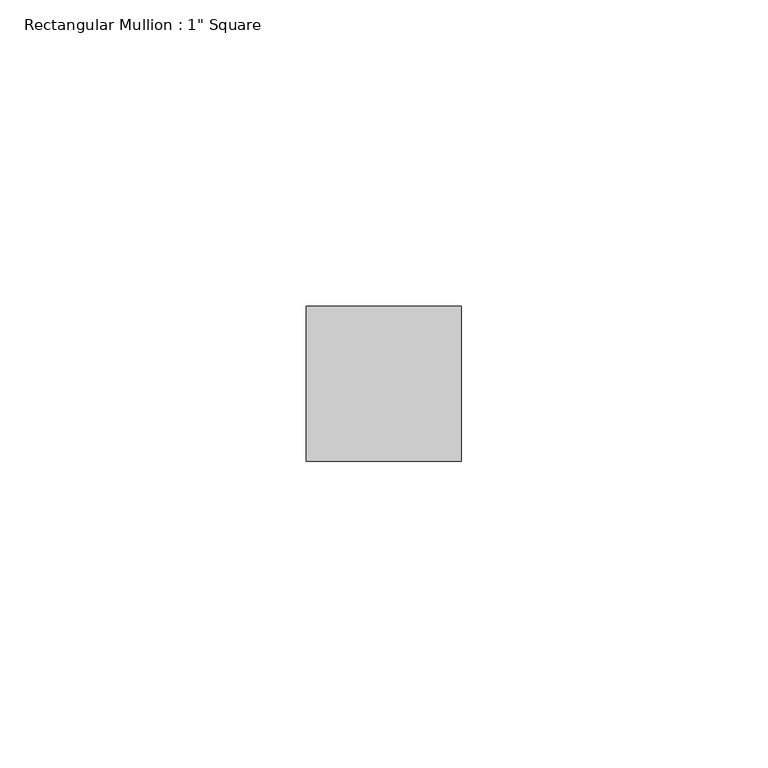
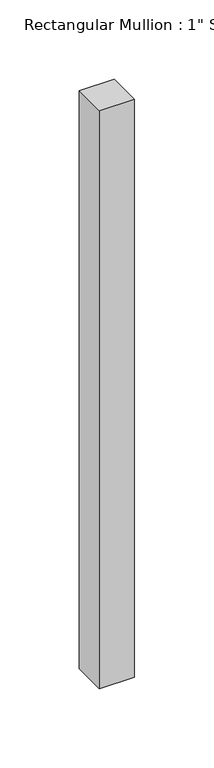
"""IFC4 building model written with IfcOpenShell, lengths in millimetres: member geometry."""

from ifc_helpers import new_model, si_unit, frame, origin, place, context, project, spatial, polyline, outline, extrude, source, transform, mapped, element, save


def member_158a8462(model_context):
    return source(origin(), model_context, "Body", "SweptSolid", [
        extrude(outline(polyline([(0.0, 12.7), (0.0, -12.7), (-25.4, -12.7), (-25.4, 12.7), (0.0, 12.7)])), frame((0.0, 0.0, -444.5), z_axis=(0.0, 0.0, 1.0), x_axis=(1.0, 0.0, 0.0)), (0.0, 0.0, 1.0), 444.5),
    ])


if __name__ == "__main__":
    model = new_model("IFC4")
    model_context = context("Model", 3, world=origin())
    ifc_project = project(units=[si_unit("LENGTHUNIT", "METRE", prefix="MILLI")], contexts=[model_context])
    site = spatial("IfcSite", under=ifc_project)
    building = spatial("IfcBuilding", under=site)
    placement = place(None, origin())
    member_shape = member_158a8462(model_context)
    element("IfcMember", 1, ObjectType="Rectangular Mullion : 1\" Square", at=placement, inside=building, context=model_context, shape_type="MappedRepresentation", body=[
        mapped(member_shape, transform((0.0, 0.0, 0.0), x_axis=(1.0, 0.0, 0.0), y_axis=(0.0, 1.0, 0.0), z_axis=(0.0, 0.0, 1.0))),
    ])
    save(model, "model.ifc")

# Revit data of these elements
# Type "Rectangular Mullion : 1\" Square"
#   built-in parameter 1007304 = 0.0833333 (stored number, unit not read)
#   built-in parameter 1007301 = 0.0416667 (stored number, unit not read)
#   built-in parameter 1007300 = 0.0416667 (stored number, unit not read)
# Element 1 (IfcMember, "Rectangular Mullion : 1\" Square")
#   Materials on its faces: "Aluminum"
# Materials
#   "Aluminum": class "Metal", colour RGB 247 247 247, transparency 0, Description = "Aluminum 6061", Cost = 0
